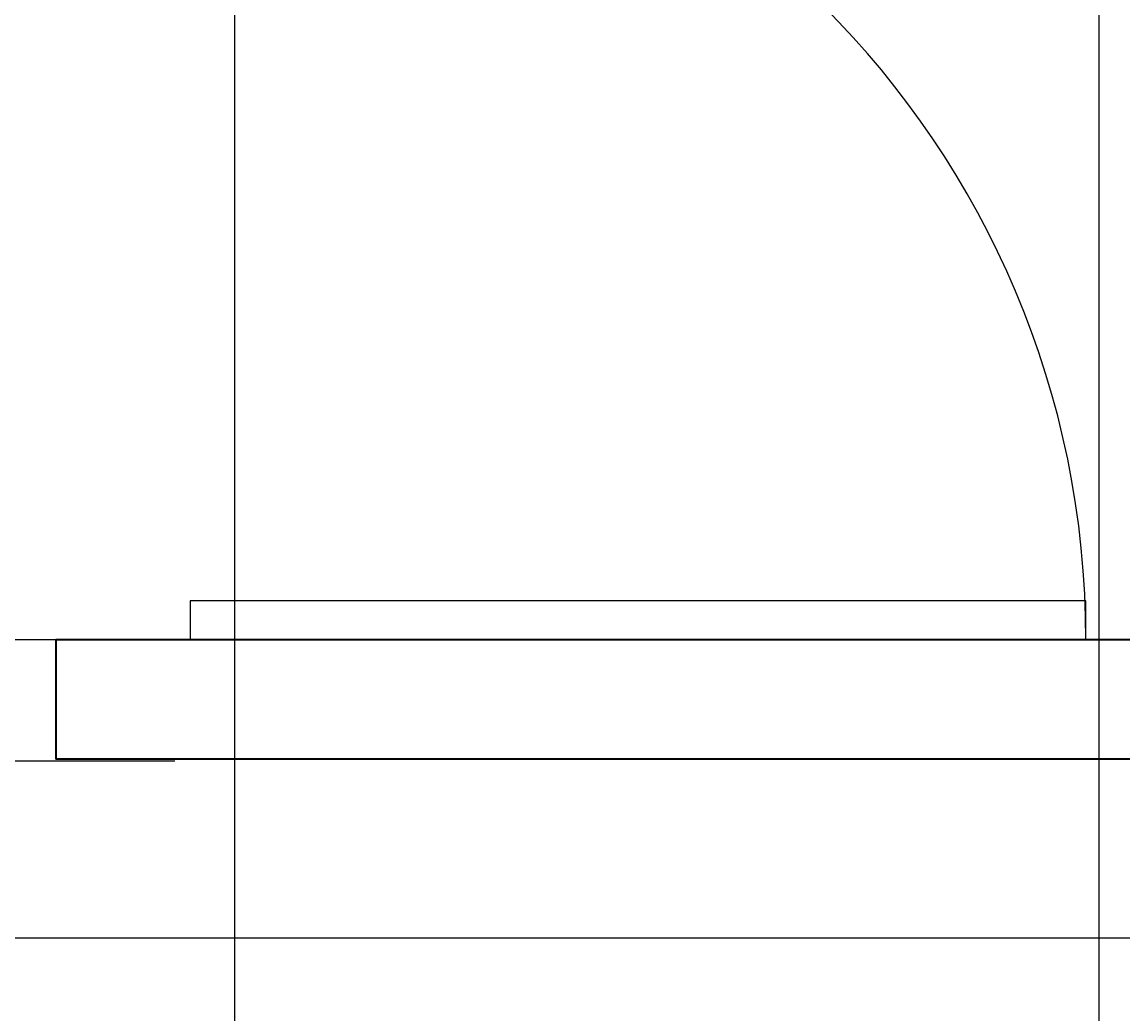
# Model space of a CAD drawing. Units: feet. Extents: x 105 to 1094, y -88 to 588.
# Tile 7 of 59: x 288 to 324, y 138 to 171. Entities that reach past the tile are written whole.
import ezdxf

# ---------------------------------------------------------------- set-up
doc = ezdxf.new("R2010")
doc.units = ezdxf.units.FT
doc.header["$MEASUREMENT"] = 0
for name, color, linetype, lineweight in [('A-ANNO-DIMS', 2, 'Continuous', 18), ('A-DOOR', 3, 'Continuous', 25), ('A-WALL', 7, 'Continuous', 35)]:
    doc.layers.add(name, color=color, linetype=linetype, lineweight=lineweight)
doc.styles.get("Standard").update_dxf_attribs({"font": 'arial.ttf'})
doc.dimstyles.get("Standard").update_dxf_attribs({"dimtxt": 0.18, "dimasz": 0.18, "dimexe": 0.18, "dimexo": 0.0625, "dimgap": 0.09, "dimtad": 0, "dimtih": 1, "dimtoh": 1, "dimdec": 4, "dimzin": 0, "dimdsep": 46, "dimtxsty": 'Standard', "dimcen": 0.09, "dimadec": 0, "dimazin": 0, "dimtfac": 1, "dimtdec": 4, "dimtofl": 0, "dimtmove": 0, "dimatfit": 3, "dimfxl": 1, "dimtolj": 1, "dimtzin": 0, "dimarcsym": 0})

# ---------------------------------------------------------------- blocks, each defined once
blk = doc.blocks.new('*U2')
blk.add_line((40, 0), (40, -6))
blk = doc.blocks.new('*U4')
for p, q in [((0, 0), (0, -6)), ((-40, 0), (-40, -6))]:
    blk.add_line(p, q)
blk.add_lwpolyline([(0, 0), (0, 40), (-1.75, 40), (-1.75, 0)], close=True)
blk.add_arc((0, 0), 40, 90, 180)
blk = doc.blocks.new('*D20')
at = {"layer": 'A-ANNO-DIMS', "color": 0, "lineweight": -2, "transparency": 16777216}
for p, q in [((150.688, 276.019), (150.688, -88.149)), ((1048.688, 276.019), (1048.688, -88.149)), ((150.868, -87.969), (599.399, -87.969)), ((1048.508, -87.969), (599.977, -87.969))]:
    blk.add_line(p, q, dxfattribs=at)
at = {"layer": 'A-ANNO-DIMS', "color": 0, "transparency": 16777216}
for points in [[(150.868, -87.939), (150.868, -87.999), (150.688, -87.969)], [(1048.508, -87.939), (1048.508, -87.999), (1048.688, -87.969)]]:
    blk.add_solid(points, dxfattribs=at)
at = {"layer": 'Defpoints', "color": 0, "transparency": 16777216}
for p in [(150.688, 276.081), (1048.688, 276.081), (1048.688, -87.969)]:
    blk.add_point(p, dxfattribs=at)
at = {"layer": 'A-ANNO-DIMS', "color": 0, "transparency": 16777216, "insert": (599.688, -87.969), "char_height": 0.18, "attachment_point": 5}
blk.add_mtext('\\A1;898', dxfattribs=at)
blk = doc.blocks.new('*D21')
at = {"layer": 'A-ANNO-DIMS', "color": 0, "lineweight": -2, "transparency": 16777216}
for p, q in [((849.626, 543.081), (105.458, 543.081)), ((105.638, 542.901), (105.638, 250.263)), ((105.638, -42.739), (105.638, 249.899)), ((849.626, -42.919), (105.458, -42.919))]:
    blk.add_line(p, q, dxfattribs=at)
at = {"layer": 'A-ANNO-DIMS', "color": 0, "transparency": 16777216}
for points in [[(105.608, 542.901), (105.668, 542.901), (105.638, 543.081)], [(105.608, -42.739), (105.668, -42.739), (105.638, -42.919)]]:
    blk.add_solid(points, dxfattribs=at)
at = {"layer": 'Defpoints', "color": 0, "transparency": 16777216}
for p in [(105.638, 543.081), (849.688, 543.081), (849.688, -42.919)]:
    blk.add_point(p, dxfattribs=at)
at = {"layer": 'A-ANNO-DIMS', "color": 0, "transparency": 16777216, "insert": (105.638, 250.081), "char_height": 0.18, "attachment_point": 5}
blk.add_mtext('\\A1;586', dxfattribs=at)
blk = doc.blocks.new('*D44')
at = {"layer": 'A-ANNO-DIMS', "color": 0, "lineweight": -2, "transparency": 16777216}
for p, q in [((294.688, 204.019), (294.688, -88.149)), ((323.688, 204.019), (323.688, -88.149)), ((294.868, -87.969), (308.968, -87.969)), ((323.508, -87.969), (309.409, -87.969))]:
    blk.add_line(p, q, dxfattribs=at)
at = {"layer": 'A-ANNO-DIMS', "color": 0, "transparency": 16777216}
for points in [[(294.868, -87.939), (294.868, -87.999), (294.688, -87.969)], [(323.508, -87.939), (323.508, -87.999), (323.688, -87.969)]]:
    blk.add_solid(points, dxfattribs=at)
at = {"layer": 'Defpoints', "color": 0, "transparency": 16777216}
for p in [(294.688, 204.081), (323.688, 204.081), (323.688, -87.969)]:
    blk.add_point(p, dxfattribs=at)
at = {"layer": 'A-ANNO-DIMS', "color": 0, "transparency": 16777216, "insert": (309.188, -87.969), "char_height": 0.18, "attachment_point": 5}
blk.add_mtext('\\A1;29', dxfattribs=at)
blk = doc.blocks.new('*D46')
at = {"layer": 'A-ANNO-DIMS', "color": 0, "lineweight": -2, "transparency": 16777216}
for p, q in [((580.626, 206.081), (105.458, 206.081)), ((105.638, 205.901), (105.638, 173.263)), ((105.638, 140.261), (105.638, 172.899)), ((580.626, 140.081), (105.458, 140.081))]:
    blk.add_line(p, q, dxfattribs=at)
at = {"layer": 'A-ANNO-DIMS', "color": 0, "transparency": 16777216}
for points in [[(105.608, 205.901), (105.668, 205.901), (105.638, 206.081)], [(105.608, 140.261), (105.668, 140.261), (105.638, 140.081)]]:
    blk.add_solid(points, dxfattribs=at)
at = {"layer": 'Defpoints', "color": 0, "transparency": 16777216}
for p in [(580.688, 206.081), (105.638, 140.081), (580.688, 140.081)]:
    blk.add_point(p, dxfattribs=at)
at = {"layer": 'A-ANNO-DIMS', "color": 0, "transparency": 16777216, "insert": (105.638, 173.081), "char_height": 0.18, "attachment_point": 5}
blk.add_mtext('\\A1;66', dxfattribs=at)
blk = doc.blocks.new('*D55')
at = {"layer": 'A-ANNO-DIMS', "color": 0, "lineweight": -2, "transparency": 16777216}
for p, q in [((292.626, 198.081), (105.458, 198.081)), ((105.638, 197.901), (105.638, 174.263)), ((105.638, 150.261), (105.638, 173.899)), ((293.134, 150.081), (105.458, 150.081))]:
    blk.add_line(p, q, dxfattribs=at)
at = {"layer": 'A-ANNO-DIMS', "color": 0, "transparency": 16777216}
for points in [[(105.608, 197.901), (105.668, 197.901), (105.638, 198.081)], [(105.608, 150.261), (105.668, 150.261), (105.638, 150.081)]]:
    blk.add_solid(points, dxfattribs=at)
at = {"layer": 'Defpoints', "color": 0, "transparency": 16777216}
for p in [(105.638, 198.081), (292.688, 198.081), (293.197, 150.081)]:
    blk.add_point(p, dxfattribs=at)
at = {"layer": 'A-ANNO-DIMS', "color": 0, "transparency": 16777216, "insert": (105.638, 174.081), "char_height": 0.18, "attachment_point": 5}
blk.add_mtext('\\A1;48', dxfattribs=at)

msp = doc.modelspace()

# ---------------------------------------------------------------- linework, layer by layer
at = {"layer": 'A-WALL'}
for p, q in [((370.6883, 150.0812), (288.6883, 150.0812)), ((288.6883, 150.0812), (288.6883, 146.0812)), ((374.6883, 146.0812), (288.6883, 146.0812))]:
    msp.add_line(p, q, dxfattribs=at)

# ---------------------------------------------------------------- block references
at = {"layer": 'A-DOOR'}
for name, p, xscale, yscale, zscale, rotation in [('*U4', (293.1967, 150.0812), 0.7513941790917756, 0.7513941790917756, 0.7513941790917756, 270), ('*U2', (287.2975, 110.0812), 0.8984622266767051, 0.8984622266767051, 0.8984622266767051, 90.00000000000003)]:
    msp.add_blockref(name, p, dxfattribs=dict(at, xscale=xscale, yscale=yscale, zscale=zscale, rotation=rotation))

# ---------------------------------------------------------------- dimensions: what is measured, and where the dimension line sits
at = {"layer": 'A-ANNO-DIMS'}
for base, p1, p2, picture, middle in [((105.6383, 543.0812), (849.6883, -42.9188), (849.6883, 543.0812), '*D21', (105.6383, 250.0812)), ((105.6383, 140.0812), (580.6883, 206.0812), (580.6883, 140.0812), '*D46', (105.6383, 173.0812)), ((105.6383, 198.0812), (293.1967, 150.0812), (292.6883, 198.0812), '*D55', (105.6383, 174.0812))]:
    dim = msp.add_linear_dim(base=base, p1=p1, p2=p2, angle=90, dimstyle='Standard', override={"dimdec": 0, "dimlfac": 1, "dimrnd": 0, "dimzin": 0, "dimdsep": 46, "dimlunit": 2}, dxfattribs=at)
    dim.commit()
    dim.dimension.update_dxf_attribs({"geometry": picture, "text_midpoint": middle})
for base, p1, p2, picture, middle in [((1048.6883, -87.9688), (150.6883, 276.0812), (1048.6883, 276.0812), '*D20', (599.6883, -87.9688)), ((323.6883, -87.9688), (294.6883, 204.0812), (323.6883, 204.0812), '*D44', (309.1883, -87.9688))]:
    dim = msp.add_linear_dim(base=base, p1=p1, p2=p2, dimstyle='Standard', override={"dimdec": 0, "dimlfac": 1, "dimrnd": 0, "dimzin": 0, "dimdsep": 46, "dimlunit": 2}, dxfattribs=at)
    dim.commit()
    dim.dimension.update_dxf_attribs({"geometry": picture, "text_midpoint": middle})

doc.saveas('drawing.dxf')
